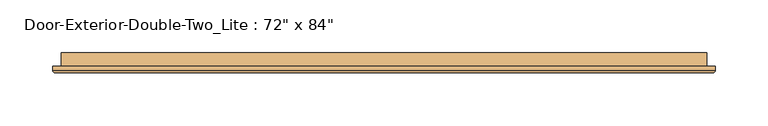
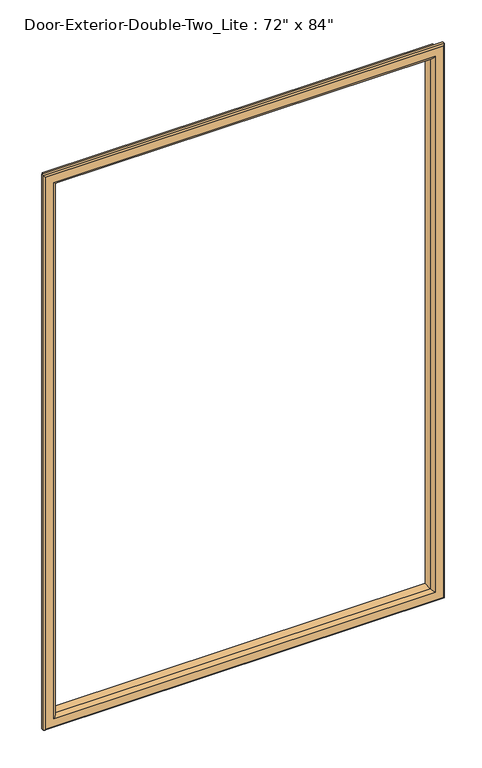
"""IFC4 building model written with IfcOpenShell, lengths in millimetres: door geometry."""

from ifc_helpers import new_model, si_unit, frame, origin, place, context, project, spatial, ellipse_curve, source, transform, mapped, element, save
from ifc_brep_helpers import plane_surface, cylinder_surface, advanced_brep


def door_95a5efb1(model_context):
    return source(origin(), model_context, "Body", "AdvancedBrep", [
        advanced_brep(
        [(-762.0, 50.8, 1117.6), (-762.0, 38.1, 1117.6), (-762.0, 38.1, 2016.125), (-762.0, 50.8, 2016.125), (-750.0, 37.1, 1129.6), (-750.0, 50.8, 1129.6), (-750.0, 50.8, 2004.125), (-750.0, 37.1, 2004.125), (-755.0, 32.1, 1124.6), (-755.0, 32.1, 2009.125), (-770.0, 34.1, 1109.6), (-768.0, 32.1, 1111.6), (-768.0, 32.1, 2022.125), (-770.0, 34.1, 2024.125), (-770.0, 38.1, 1109.6), (-770.0, 38.1, 2024.125), (-152.4, 38.1, 2016.125), (-152.4, 50.8, 2016.125), (-164.4, 50.8, 2004.125), (-164.4, 37.1, 2004.125), (-159.4, 32.1, 2009.125), (-146.4, 32.1, 2022.125), (-144.4, 34.1, 2024.125), (-144.4, 38.1, 2024.125), (-152.4, 38.1, 1117.6), (-152.4, 50.8, 1117.6), (-164.4, 50.8, 1129.6), (-164.4, 37.1, 1129.6), (-159.4, 32.1, 1124.6), (-146.4, 32.1, 1111.6), (-144.4, 34.1, 1109.6), (-144.4, 38.1, 1109.6)],
        [
            (0, 1),
            (1, 2),
            (2, 3),
            (3, 0),
            (4, 5),
            (5, 6),
            (6, 7),
            (7, 4),
            (8, 4, ellipse_curve(frame((-755.0, 37.1, 1124.6), z_axis=(-0.7071067811865475, 0.0, 0.7071067811865475), x_axis=(-0.7071067811865474, 0.0, -0.7071067811865476)), 7.0710678, 5.0)),
            (7, 9, ellipse_curve(frame((-755.0, 37.1, 2009.125), z_axis=(-0.7071067811865475, 0.0, -0.7071067811865475), x_axis=(0.7071067811865474, 0.0, -0.7071067811865476)), 7.0710678, 5.0)),
            (9, 8),
            (10, 11, ellipse_curve(frame((-768.0, 34.1, 1111.6), z_axis=(-0.7071067811865475, 0.0, 0.7071067811865475), x_axis=(-0.7071067811865474, 0.0, -0.7071067811865476)), 2.8284271, 2.0)),
            (11, 12),
            (12, 13, ellipse_curve(frame((-768.0, 34.1, 2022.125), z_axis=(-0.7071067811865475, 0.0, -0.7071067811865475), x_axis=(0.7071067811865474, 0.0, -0.7071067811865476)), 2.8284271, 2.0)),
            (13, 10),
            (14, 10),
            (13, 15),
            (15, 14),
            (2, 16),
            (16, 17),
            (17, 3),
            (6, 18),
            (18, 19),
            (19, 7),
            (19, 20, ellipse_curve(frame((-159.4, 37.1, 2009.125), z_axis=(-0.7071067811865475, 0.0, 0.7071067811865475), x_axis=(-0.7071067811865476, 0.0, -0.7071067811865474)), 7.0710678, 5.0)),
            (20, 9),
            (12, 21),
            (21, 22, ellipse_curve(frame((-146.4, 34.1, 2022.125), z_axis=(-0.7071067811865475, 0.0, 0.7071067811865475), x_axis=(-0.7071067811865476, 0.0, -0.7071067811865474)), 2.8284271, 2.0)),
            (22, 13),
            (22, 23),
            (23, 15),
            (16, 24),
            (24, 25),
            (25, 17),
            (18, 26),
            (26, 27),
            (27, 19),
            (27, 28, ellipse_curve(frame((-159.4, 37.1, 1124.6), z_axis=(0.7071067811865475, 0.0, 0.7071067811865475), x_axis=(-0.7071067811865474, 0.0, 0.7071067811865476)), 7.0710678, 5.0)),
            (28, 20),
            (21, 29),
            (29, 30, ellipse_curve(frame((-146.4, 34.1, 1111.6), z_axis=(0.7071067811865475, 0.0, 0.7071067811865475), x_axis=(-0.7071067811865474, 0.0, 0.7071067811865476)), 2.8284271, 2.0)),
            (30, 22),
            (30, 31),
            (31, 23),
            (31, 14),
            (1, 24),
            (0, 25),
            (5, 26),
            (4, 27),
            (8, 28),
            (11, 29),
            (10, 30),
        ],
        [
            plane_surface(frame((-762.0, 38.1, 1117.6), z_axis=(-1.0, 0.0, 0.0), x_axis=(0.0, 0.0, 1.0))),
            plane_surface(frame((-750.0, 50.8, 1129.6), z_axis=(1.0, 0.0, 0.0), x_axis=(0.0, 0.0, 1.0))),
            cylinder_surface(frame((-755.0, 37.1, 1117.6), z_axis=(0.0, 0.0, -1.0), x_axis=(-1.0, 0.0, 0.0)), 5.0),
            cylinder_surface(frame((-768.0, 34.1, 1117.6), z_axis=(0.0, 0.0, -1.0), x_axis=(-1.0, 0.0, 0.0)), 2.0),
            plane_surface(frame((-770.0, 34.1, 1109.6), z_axis=(-1.0, 0.0, 0.0), x_axis=(0.0, 0.0, 1.0))),
            plane_surface(frame((-762.0, 38.1, 2016.125), z_axis=(0.0, 0.0, 1.0), x_axis=(1.0, 0.0, 0.0))),
            plane_surface(frame((-750.0, 50.8, 2004.125), z_axis=(0.0, 0.0, -1.0), x_axis=(1.0, 0.0, 0.0))),
            cylinder_surface(frame((-762.0, 37.1, 2009.125), z_axis=(-1.0, 0.0, 0.0), x_axis=(0.0, 0.0, 1.0)), 5.0),
            cylinder_surface(frame((-762.0, 34.1, 2022.125), z_axis=(-1.0, 0.0, 0.0), x_axis=(0.0, 0.0, 1.0)), 2.0),
            plane_surface(frame((-770.0, 34.1, 2024.125), z_axis=(0.0, 0.0, 1.0), x_axis=(1.0, 0.0, 0.0))),
            plane_surface(frame((-152.4, 38.1, 2016.125), z_axis=(1.0, 0.0, 0.0), x_axis=(0.0, 0.0, -1.0))),
            plane_surface(frame((-164.4, 50.8, 2004.125), z_axis=(-1.0, 0.0, 0.0), x_axis=(0.0, 0.0, -1.0))),
            cylinder_surface(frame((-159.4, 37.1, 2016.125), z_axis=(0.0, 0.0, 1.0), x_axis=(1.0, 0.0, 0.0)), 5.0),
            cylinder_surface(frame((-146.4, 34.1, 2016.125), z_axis=(0.0, 0.0, 1.0), x_axis=(1.0, 0.0, 0.0)), 2.0),
            plane_surface(frame((-144.4, 34.1, 2024.125), z_axis=(1.0, 0.0, 0.0), x_axis=(0.0, 0.0, -1.0))),
            plane_surface(frame((-144.4, 38.1, 1109.6), z_axis=(0.0, 1.0, 0.0), x_axis=(-1.0, 0.0, 0.0))),
            plane_surface(frame((-152.4, 38.1, 1117.6), z_axis=(0.0, 0.0, -1.0), x_axis=(-1.0, 0.0, 0.0))),
            plane_surface(frame((-152.4, 50.8, 1117.6), z_axis=(0.0, 1.0, 0.0), x_axis=(-1.0, 0.0, 0.0))),
            plane_surface(frame((-164.4, 50.8, 1129.6), z_axis=(0.0, 0.0, 1.0), x_axis=(-1.0, 0.0, 0.0))),
            cylinder_surface(frame((-152.4, 37.1, 1124.6), z_axis=(1.0, 0.0, 0.0), x_axis=(0.0, 0.0, -1.0)), 5.0),
            plane_surface(frame((-159.4, 32.1, 1124.6), z_axis=(0.0, -1.0, 0.0), x_axis=(-1.0, 0.0, 0.0))),
            cylinder_surface(frame((-152.4, 34.1, 1111.6), z_axis=(1.0, 0.0, 0.0), x_axis=(0.0, 0.0, -1.0)), 2.0),
            plane_surface(frame((-144.4, 34.1, 1109.6), z_axis=(0.0, 0.0, -1.0), x_axis=(-1.0, 0.0, 0.0))),
        ],
        [
            (0, [[1, 2, 3, 4]]),
            (1, [[5, 6, 7, 8]]),
            (2, [[9, -8, 10, 11]]),
            (3, [[12, 13, 14, 15]]),
            (4, [[16, -15, 17, 18]]),
            (5, [[-3, 19, 20, 21]]),
            (6, [[-7, 22, 23, 24]]),
            (7, [[-10, -24, 25, 26]]),
            (8, [[-14, 27, 28, 29]]),
            (9, [[-17, -29, 30, 31]]),
            (10, [[-20, 32, 33, 34]]),
            (11, [[-23, 35, 36, 37]]),
            (12, [[-25, -37, 38, 39]]),
            (13, [[-28, 40, 41, 42]]),
            (14, [[-30, -42, 43, 44]]),
            (15, [[-31, -44, 45, -18], [46, -32, -19, -2]]),
            (16, [[-33, -46, -1, 47]]),
            (17, [[-21, -34, -47, -4], [48, -35, -22, -6]]),
            (18, [[-36, -48, -5, 49]]),
            (19, [[-38, -49, -9, 50]]),
            (20, [[51, -40, -27, -13], [-26, -39, -50, -11]]),
            (21, [[-41, -51, -12, 52]]),
            (22, [[-43, -52, -16, -45]]),
        ],
    ),
    ])


if __name__ == "__main__":
    model = new_model("IFC4")
    model_context = context("Model", 3, world=origin())
    ifc_project = project(units=[si_unit("LENGTHUNIT", "METRE", prefix="MILLI")], contexts=[model_context])
    site = spatial("IfcSite", under=ifc_project)
    building = spatial("IfcBuilding", under=site)
    placement = place(None, origin())
    door_shape = door_95a5efb1(model_context)
    element("IfcDoor", 1, ObjectType="Door-Exterior-Double-Two_Lite : 72\" x 84\"", at=placement, inside=building, context=model_context, shape_type="MappedRepresentation", body=[
        mapped(door_shape, transform((0.0, 0.0, 0.0), x_axis=(1.0, 0.0, 0.0), y_axis=(0.0, 1.0, 0.0), z_axis=(0.0, 0.0, 1.0))),
    ])
    save(model, "model.ifc")

# Revit data of these elements
# Type "Door-Exterior-Double-Two_Lite : 72\" x 84\""
#   Type Mark = "8"
#   Assembly Code = "B2030100"
#   Analytic Construction = "Metal frame, double glass door"
#   Top Rail = 0' - 4 5/8"
#   Threshold Length [instance default] = 6' - 4"
#   Threshold Offset [instance default] = 0' - 0 1/2"
#   Thickness = 0' - 1 3/4"
#   Thermal Resistance (R) = 1.3794 (h·ft²·°F)/BTU
#   Swing Angle [instance default] = 90.00°
#   Strike Height = 3' - 4"
#   Stiles = 0' - 6"
#   SinglePanelWidth = 3' - 0"
#   Rough Width [instance default] = 6' - 4"
#   Rough Height [instance default] = 7' - 4"
#   MFOpeningHeight [instance default] = 0' - 4"
#   MFOpeningWidth [instance default] = 0' - 4"
#   Lock Rail = 0' - 8"
#   Inset Calculate [instance default] = 0' - 4"
#   Masonry Inset [instance default] = 0' - 1"
#   Height = 7' - 0"
#   Width = 6' - 0"
#   Heat Transfer Coefficient (U) = 0.7250 BTU/(h·ft²·°F)
#   Glass Thickness = 0' - 0 3/4"
#   Masonry Frame Depth = 0' - 5 3/4"
#   Bottom Rail = 0' - 10"
#   Threshold [instance default] = yes
#   Masonry Frame [instance default] = yes
#   Function = 1
#   Dry Wall Frame [instance default] = no
#   Threshold Material = none
#   Panic Bar Material = Metal - Stainless Steel
#   Panel Material = Metal - Painted - Grey
#   Glass Stop Material = Metal - Painted - Grey
#   Frame Material = Metal - Painted - Grey
#   Exterior Pull Material = Metal - Stainless Steel
#   Visual Light Transmittance = 0
#   Solar Heat Gain Coefficient = 0
#   Wall Closure = (empty or 0)
# Element 1 (IfcDoor, "Door-Exterior-Double-Two_Lite : 72\" x 84\"")
#   Materials on its faces: "Metal - Painted - Grey", "Metal - Stainless Steel", "Glass"
# Materials
#   "Metal - Stainless Steel": class "Metal", colour RGB 247 247 247, transparency 0
#   "Metal - Painted - Grey": class "Paint", colour RGB 104 104 104, transparency 0, Cost = 0
#   "Glass": class "Glass", colour RGB 0 128 192, transparency 0.75, Description = "Soda Lime Glass", Cost = 0
